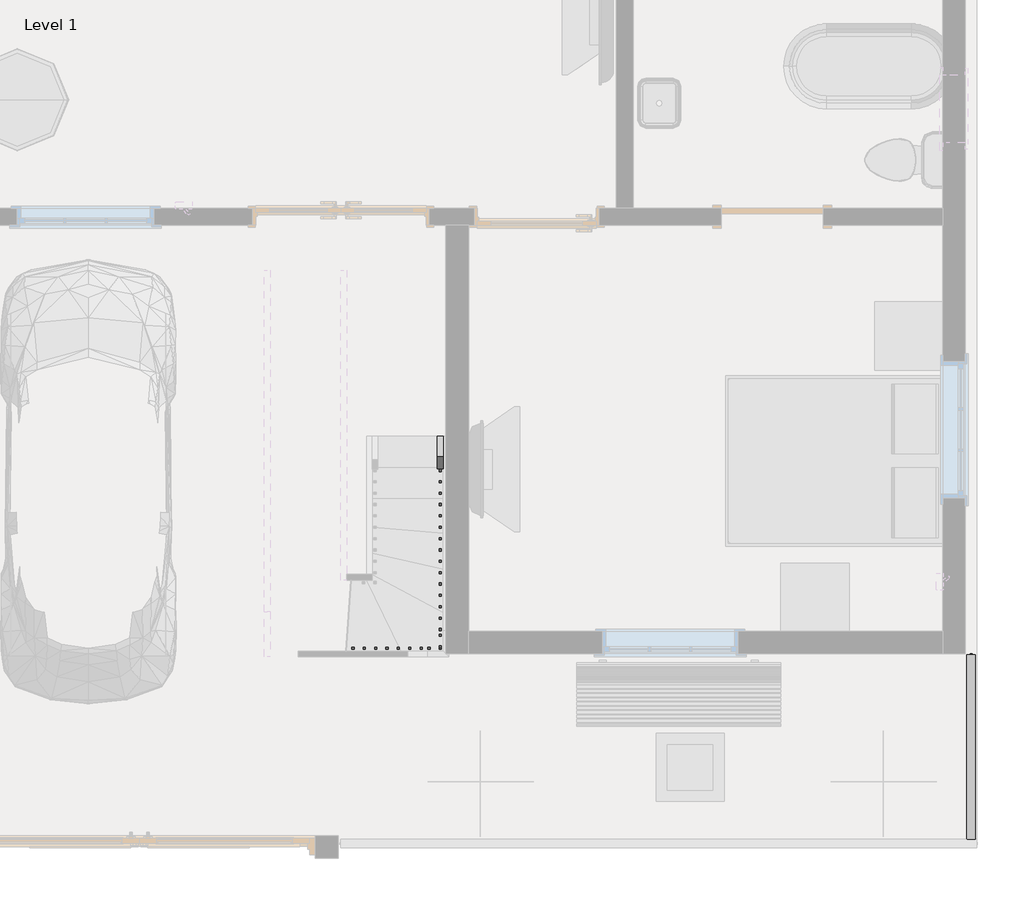
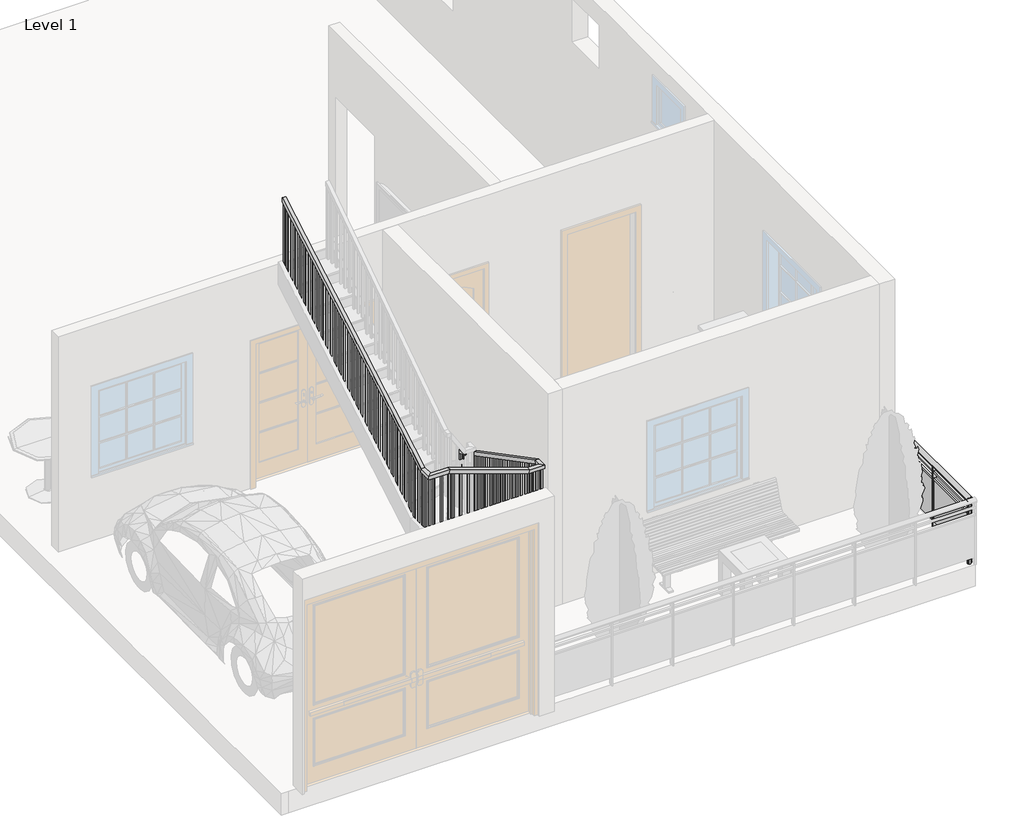
# One storey, part 2 of 3: 2 railings.
"""IFC4 building model written with IfcOpenShell, lengths in millimetres."""

from ifc_helpers import new_model, si_unit, point, frame, origin, origin_with_axes, place, context, project, spatial, polyline, ellipse_curve, trimmed, outline, extrude, faceted_brep, element, save
from ifc_brep_helpers import plane_surface, extruded_surface, advanced_brep

model = new_model("IFC4")

# Units and contexts
model_context = context("Model", 3, world=origin())
ifc_project = project(units=[si_unit("LENGTHUNIT", "METRE", prefix="MILLI")], contexts=[model_context])

# Site, building, storey
site = spatial("IfcSite", under=ifc_project)
building = spatial("IfcBuilding", under=site)
storey = spatial("IfcBuildingStorey", under=building, Name="Level 1", Elevation=0.0)

# Railings
placement = place(None, origin())
element("IfcRailing", 1, ObjectType="Glass Panel - Bottom Fill", at=placement, inside=storey, context=model_context, shape_type="SolidModel", body=[
    advanced_brep(
    [(-6322.409927, -1583.0384156, 914.4), (-6246.209927, -1583.0384156, 914.4), (-6322.409927, 67.9615844, 914.4), (-6246.209927, 67.9615844, 914.4)],
    [
        (0, 1, ellipse_curve(frame((-6284.309927, -1583.0384156, 914.4), z_axis=(0.0, -1.0, 0.0), x_axis=(1.0, 0.0, 0.0)), 38.1, 28.575)),
        (1, 0, ellipse_curve(frame((-6284.309927, -1583.0384156, 914.4), z_axis=(0.0, -1.0, 0.0), x_axis=(1.0, 0.0, 0.0)), 38.1, 28.575)),
        (2, 3, ellipse_curve(frame((-6284.309927, 67.9615844, 914.4), z_axis=(0.0, 1.0, 0.0), x_axis=(1.0, 0.0, 0.0)), 38.1, 28.575)),
        (3, 2, ellipse_curve(frame((-6284.309927, 67.9615844, 914.4), z_axis=(0.0, 1.0, 0.0), x_axis=(1.0, 0.0, 0.0)), 38.1, 28.575)),
        (0, 2),
        (3, 1),
    ],
    [
        plane_surface(frame((-6284.309927, -1583.0384156, 914.4), z_axis=(0.0, -1.0, 0.0), x_axis=(0.0, 0.0, 1.0))),
        plane_surface(frame((-6284.309927, 67.9615844, 914.4), z_axis=(0.0, 1.0, 0.0), x_axis=(0.0, 0.0, 1.0))),
        extruded_surface(trimmed(ellipse_curve(frame((-6284.309927, 67.9615844, 914.4), z_axis=(0.0, -1.0, 0.0), x_axis=(1.0, 0.0, 0.0)), 38.1, 28.575), [point((-6322.409927, 67.9615844, 914.4))], [point((-6246.209927, 67.9615844, 914.4))], True, "CARTESIAN"), (0.0, -1651.0, 0.0), 1651.0),
        extruded_surface(trimmed(ellipse_curve(frame((-6284.309927, 67.9615844, 914.4), z_axis=(0.0, -1.0, 0.0), x_axis=(1.0, 0.0, 0.0)), 38.1, 28.575), [point((-6246.209927, 67.9615844, 914.4))], [point((-6322.409927, 67.9615844, 914.4))], True, "CARTESIAN"), (0.0, -1651.0, 0.0), 1651.0),
    ],
    [
        (0, [[1, 2]]),
        (1, [[3, 4]]),
        (2, [[-1, 5, -4, 6]]),
        (3, [[-2, -6, -3, -5]]),
    ],
),
    extrude(outline(polyline([(-6271.609927, -1583.0384156), (-6297.009927, -1583.0384156), (-6297.009927, 67.9615844), (-6271.609927, 67.9615844), (-6271.609927, -1583.0384156)])), frame((0.0, 0.0, 800.1), z_axis=(0.0, 0.0, 1.0), x_axis=(1.0, 0.0, 0.0)), (0.0, 0.0, 1.0), 25.4),
    extrude(outline(polyline([(-6271.609927, -1583.0384156), (-6297.009927, -1583.0384156), (-6297.009927, 67.9615844), (-6271.609927, 67.9615844), (-6271.609927, -1583.0384156)])), frame((0.0, 0.0, 698.5), z_axis=(0.0, 0.0, 1.0), x_axis=(1.0, 0.0, 0.0)), (0.0, 0.0, 1.0), 25.4),
    extrude(outline(polyline([(-6258.909927, 48.9115844), (-6309.709927, 48.9115844), (-6309.709927, 61.6115844), (-6258.909927, 61.6115844), (-6258.909927, 48.9115844)])), origin_with_axes(), (0.0, 0.0, 1.0), 885.6788223),
    extrude(outline(polyline([(-6290.845084, -757.5384156), (-6290.845084, 55.2615844), (-6284.495084, 55.2615844), (-6284.495084, -757.5384156), (-6290.845084, -757.5384156)])), frame((0.0, 0.0, 101.6), z_axis=(0.0, 0.0, 1.0), x_axis=(1.0, 0.0, 0.0)), (0.0, 0.0, 1.0), 596.9),
    extrude(outline(polyline([(-6258.909927, -763.8884156), (-6309.709927, -763.8884156), (-6309.709927, -751.1884156), (-6258.909927, -751.1884156), (-6258.909927, -763.8884156)])), origin_with_axes(), (0.0, 0.0, 1.0), 885.6788223),
    extrude(outline(polyline([(-6290.845084, -1570.3384156), (-6290.845084, -757.5384156), (-6284.495084, -757.5384156), (-6284.495084, -1570.3384156), (-6290.845084, -1570.3384156)])), frame((0.0, 0.0, 101.6), z_axis=(0.0, 0.0, 1.0), x_axis=(1.0, 0.0, 0.0)), (0.0, 0.0, 1.0), 596.9),
    extrude(outline(polyline([(-6258.909927, -1576.6884156), (-6309.709927, -1576.6884156), (-6309.709927, -1563.9884156), (-6258.909927, -1563.9884156), (-6258.909927, -1576.6884156)])), origin_with_axes(), (0.0, 0.0, 1.0), 885.6788223),
    extrude(outline(polyline([(-6274.784927, 55.2615844), (-6293.834927, 55.2615844), (-6293.834927, 74.3115844), (-6274.784927, 74.3115844), (-6274.784927, 55.2615844)])), origin_with_axes(), (0.0, 0.0, 1.0), 885.6788223),
    extrude(outline(polyline([(-6274.784927, -1589.3884156), (-6293.834927, -1589.3884156), (-6293.834927, -1570.3384156), (-6274.784927, -1570.3384156), (-6274.784927, -1589.3884156)])), origin_with_axes(), (0.0, 0.0, 1.0), 885.6788223),
])
element("IfcRailing", 2, ObjectType="Handrail - Rectangular", at=placement, inside=storey, context=model_context, shape_type="SolidModel", body=[
    faceted_brep([(-11008.709927, 2021.0747681, 1107.1884661), (-11008.709927, 2021.0747681, 1049.8811723), (-11059.509927, 2021.0747681, 1049.8811723), (-11059.509927, 2021.0747681, 1107.1884661), (-11008.709927, 241.9248873, 2036.1046546), (-11008.709927, 229.4614905, 1985.3046546), (-11059.509927, 229.4614905, 1985.3046546), (-11059.509927, 241.9248873, 2036.1046546), (-11008.709927, 100.7187882, 2036.1046546), (-11008.709927, 100.7187882, 1985.3046546), (-11059.509927, 151.5187882, 1985.3046546), (-11059.509927, 151.5187882, 2036.1046546), (-11205.9185931, 100.7187882, 2036.1046546), (-11214.5966373, 100.7187882, 1985.3046546), (-11214.5966373, 151.5187882, 1985.3046546), (-11205.9185931, 151.5187882, 2036.1046546), (-12274.7947104, 100.7187882, 2412.269093), (-12283.4727547, 100.7187882, 2361.469093), (-12283.4727547, 151.5187882, 2361.469093), (-12274.7947104, 151.5187882, 2412.269093), (-12558.109927, 100.7187882, 2412.269093), (-12558.109927, 100.7187882, 2361.469093), (-12507.309927, 151.5187882, 2361.469093), (-12507.309927, 151.5187882, 2412.269093), (-12558.109927, 281.7971454, 2412.269093), (-12558.109927, 295.524936, 2361.469093), (-12507.309927, 295.524936, 2361.469093), (-12507.309927, 281.7971454, 2412.269093), (-12558.109927, 3510.3281176, 4294.6349858), (-12507.309927, 3510.3281176, 4294.6349858), (-12507.309927, 3510.3281176, 4235.8311212), (-12558.109927, 3510.3281176, 4235.8311212)], [[[0, 1, 2, 3]], [[1, 0, 4, 5]], [[2, 1, 5, 6]], [[3, 2, 6, 7]], [[0, 3, 7, 4]], [[5, 4, 8, 9]], [[6, 5, 9, 10]], [[7, 6, 10, 11]], [[4, 7, 11, 8]], [[9, 8, 12, 13]], [[10, 9, 13, 14]], [[11, 10, 14, 15]], [[8, 11, 15, 12]], [[13, 12, 16, 17]], [[14, 13, 17, 18]], [[15, 14, 18, 19]], [[12, 15, 19, 16]], [[17, 16, 20, 21]], [[18, 17, 21, 22]], [[19, 18, 22, 23]], [[16, 19, 23, 20]], [[21, 20, 24, 25]], [[22, 21, 25, 26]], [[23, 22, 26, 27]], [[20, 23, 27, 24]], [[28, 29, 30, 31]], [[25, 24, 28, 31]], [[26, 25, 31, 30]], [[27, 26, 30, 29]], [[24, 27, 29, 28]]]),
    extrude(outline(polyline([(3440.9221454, 4195.3645945), (3440.9221454, 3217.3333333), (3421.8721454, 3217.3333333), (3421.8721454, 4184.2576637), (3440.9221454, 4195.3645945)])), frame((-12542.234927, 0.0, 0.0), z_axis=(1.0, 0.0, 0.0), x_axis=(0.0, 1.0, 0.0)), (0.0, 0.0, 1.0), 19.05),
    extrude(outline(polyline([(3339.3221454, 4136.12763), (3339.3221454, 3217.3333333), (3320.2721454, 3217.3333333), (3320.2721454, 4125.0206991), (3339.3221454, 4136.12763)])), frame((-12542.234927, 0.0, 0.0), z_axis=(1.0, 0.0, 0.0), x_axis=(0.0, 1.0, 0.0)), (0.0, 0.0, 1.0), 19.05),
    extrude(outline(polyline([(3237.7221454, 4076.8906654), (3237.7221454, 3048.0), (3218.6721454, 3048.0), (3218.6721454, 4065.7837346), (3237.7221454, 4076.8906654)])), frame((-12542.234927, 0.0, 0.0), z_axis=(1.0, 0.0, 0.0), x_axis=(0.0, 1.0, 0.0)), (0.0, 0.0, 1.0), 19.05),
    extrude(outline(polyline([(3136.1221454, 4017.6537009), (3136.1221454, 3048.0), (3117.0721454, 3048.0), (3117.0721454, 4006.5467701), (3136.1221454, 4017.6537009)])), frame((-12542.234927, 0.0, 0.0), z_axis=(1.0, 0.0, 0.0), x_axis=(0.0, 1.0, 0.0)), (0.0, 0.0, 1.0), 19.05),
    extrude(outline(polyline([(3034.5221454, 3958.4167364), (3034.5221454, 3048.0), (3015.4721454, 3048.0), (3015.4721454, 3947.3098055), (3034.5221454, 3958.4167364)])), frame((-12542.234927, 0.0, 0.0), z_axis=(1.0, 0.0, 0.0), x_axis=(0.0, 1.0, 0.0)), (0.0, 0.0, 1.0), 19.05),
    extrude(outline(polyline([(2932.9221454, 3899.1797718), (2932.9221454, 2878.6666667), (2913.8721454, 2878.6666667), (2913.8721454, 3888.072841), (2932.9221454, 3899.1797718)])), frame((-12542.234927, 0.0, 0.0), z_axis=(1.0, 0.0, 0.0), x_axis=(0.0, 1.0, 0.0)), (0.0, 0.0, 1.0), 19.05),
    extrude(outline(polyline([(2831.3221454, 3839.9428073), (2831.3221454, 2878.6666667), (2812.2721454, 2878.6666667), (2812.2721454, 3828.8358764), (2831.3221454, 3839.9428073)])), frame((-12542.234927, 0.0, 0.0), z_axis=(1.0, 0.0, 0.0), x_axis=(0.0, 1.0, 0.0)), (0.0, 0.0, 1.0), 19.05),
    extrude(outline(polyline([(2729.7221454, 3780.7058428), (2729.7221454, 2878.6666667), (2710.6721454, 2878.6666667), (2710.6721454, 3769.5989119), (2729.7221454, 3780.7058428)])), frame((-12542.234927, 0.0, 0.0), z_axis=(1.0, 0.0, 0.0), x_axis=(0.0, 1.0, 0.0)), (0.0, 0.0, 1.0), 19.05),
    extrude(outline(polyline([(2628.1221454, 3721.4688782), (2628.1221454, 2709.3333333), (2609.0721454, 2709.3333333), (2609.0721454, 3710.3619474), (2628.1221454, 3721.4688782)])), frame((-12542.234927, 0.0, 0.0), z_axis=(1.0, 0.0, 0.0), x_axis=(0.0, 1.0, 0.0)), (0.0, 0.0, 1.0), 19.05),
    extrude(outline(polyline([(2526.5221454, 3662.2319137), (2526.5221454, 2709.3333333), (2507.4721454, 2709.3333333), (2507.4721454, 3651.1249828), (2526.5221454, 3662.2319137)])), frame((-12542.234927, 0.0, 0.0), z_axis=(1.0, 0.0, 0.0), x_axis=(0.0, 1.0, 0.0)), (0.0, 0.0, 1.0), 19.05),
    extrude(outline(polyline([(2424.9221454, 3602.9949491), (2424.9221454, 2709.3333333), (2405.8721454, 2709.3333333), (2405.8721454, 3591.8880183), (2424.9221454, 3602.9949491)])), frame((-12542.234927, 0.0, 0.0), z_axis=(1.0, 0.0, 0.0), x_axis=(0.0, 1.0, 0.0)), (0.0, 0.0, 1.0), 19.05),
    extrude(outline(polyline([(2323.3221454, 3543.7579846), (2323.3221454, 2540.0), (2304.2721454, 2540.0), (2304.2721454, 3532.6510537), (2323.3221454, 3543.7579846)])), frame((-12542.234927, 0.0, 0.0), z_axis=(1.0, 0.0, 0.0), x_axis=(0.0, 1.0, 0.0)), (0.0, 0.0, 1.0), 19.05),
    extrude(outline(polyline([(2221.7221454, 3484.5210201), (2221.7221454, 2540.0), (2202.6721454, 2540.0), (2202.6721454, 3473.4140892), (2221.7221454, 3484.5210201)])), frame((-12542.234927, 0.0, 0.0), z_axis=(1.0, 0.0, 0.0), x_axis=(0.0, 1.0, 0.0)), (0.0, 0.0, 1.0), 19.05),
    extrude(outline(polyline([(2120.1221454, 3425.2840555), (2120.1221454, 2540.0), (2101.0721454, 2540.0), (2101.0721454, 3414.1771247), (2120.1221454, 3425.2840555)])), frame((-12542.234927, 0.0, 0.0), z_axis=(1.0, 0.0, 0.0), x_axis=(0.0, 1.0, 0.0)), (0.0, 0.0, 1.0), 19.05),
    extrude(outline(polyline([(2018.5221454, 3366.047091), (2018.5221454, 2370.6666667), (1999.4721454, 2370.6666667), (1999.4721454, 3354.9401601), (2018.5221454, 3366.047091)])), frame((-12542.234927, 0.0, 0.0), z_axis=(1.0, 0.0, 0.0), x_axis=(0.0, 1.0, 0.0)), (0.0, 0.0, 1.0), 19.05),
    extrude(outline(polyline([(1916.9221454, 3306.8101264), (1916.9221454, 2370.6666667), (1897.8721454, 2370.6666667), (1897.8721454, 3295.7031956), (1916.9221454, 3306.8101264)])), frame((-12542.234927, 0.0, 0.0), z_axis=(1.0, 0.0, 0.0), x_axis=(0.0, 1.0, 0.0)), (0.0, 0.0, 1.0), 19.05),
    extrude(outline(polyline([(1815.3221454, 3247.5731619), (1815.3221454, 2201.3333333), (1796.2721454, 2201.3333333), (1796.2721454, 3236.466231), (1815.3221454, 3247.5731619)])), frame((-12542.234927, 0.0, 0.0), z_axis=(1.0, 0.0, 0.0), x_axis=(0.0, 1.0, 0.0)), (0.0, 0.0, 1.0), 19.05),
    extrude(outline(polyline([(1713.7221454, 3188.3361974), (1713.7221454, 2201.3333333), (1694.6721454, 2201.3333333), (1694.6721454, 3177.2292665), (1713.7221454, 3188.3361974)])), frame((-12542.234927, 0.0, 0.0), z_axis=(1.0, 0.0, 0.0), x_axis=(0.0, 1.0, 0.0)), (0.0, 0.0, 1.0), 19.05),
    extrude(outline(polyline([(1612.1221454, 3129.0992328), (1612.1221454, 2201.3333333), (1593.0721454, 2201.3333333), (1593.0721454, 3117.992302), (1612.1221454, 3129.0992328)])), frame((-12542.234927, 0.0, 0.0), z_axis=(1.0, 0.0, 0.0), x_axis=(0.0, 1.0, 0.0)), (0.0, 0.0, 1.0), 19.05),
    extrude(outline(polyline([(1510.5221454, 3069.8622683), (1510.5221454, 2032.0), (1491.4721454, 2032.0), (1491.4721454, 3058.7553374), (1510.5221454, 3069.8622683)])), frame((-12542.234927, 0.0, 0.0), z_axis=(1.0, 0.0, 0.0), x_axis=(0.0, 1.0, 0.0)), (0.0, 0.0, 1.0), 19.05),
    extrude(outline(polyline([(1408.9221454, 3010.6253037), (1408.9221454, 2032.0), (1389.8721454, 2032.0), (1389.8721454, 2999.5183729), (1408.9221454, 3010.6253037)])), frame((-12542.234927, 0.0, 0.0), z_axis=(1.0, 0.0, 0.0), x_axis=(0.0, 1.0, 0.0)), (0.0, 0.0, 1.0), 19.05),
    extrude(outline(polyline([(1307.3221454, 2951.3883392), (1307.3221454, 2032.0), (1288.2721454, 2032.0), (1288.2721454, 2940.2814083), (1307.3221454, 2951.3883392)])), frame((-12542.234927, 0.0, 0.0), z_axis=(1.0, 0.0, 0.0), x_axis=(0.0, 1.0, 0.0)), (0.0, 0.0, 1.0), 19.05),
    extrude(outline(polyline([(1205.7221454, 2892.1513747), (1205.7221454, 1862.6666667), (1186.6721454, 1862.6666667), (1186.6721454, 2881.0444438), (1205.7221454, 2892.1513747)])), frame((-12542.234927, 0.0, 0.0), z_axis=(1.0, 0.0, 0.0), x_axis=(0.0, 1.0, 0.0)), (0.0, 0.0, 1.0), 19.05),
    extrude(outline(polyline([(1104.1221454, 2832.9144101), (1104.1221454, 1862.6666667), (1085.0721454, 1862.6666667), (1085.0721454, 2821.8074793), (1104.1221454, 2832.9144101)])), frame((-12542.234927, 0.0, 0.0), z_axis=(1.0, 0.0, 0.0), x_axis=(0.0, 1.0, 0.0)), (0.0, 0.0, 1.0), 19.05),
    extrude(outline(polyline([(1002.5221454, 2773.6774456), (1002.5221454, 1862.6666667), (983.4721454, 1862.6666667), (983.4721454, 2762.5705147), (1002.5221454, 2773.6774456)])), frame((-12542.234927, 0.0, 0.0), z_axis=(1.0, 0.0, 0.0), x_axis=(0.0, 1.0, 0.0)), (0.0, 0.0, 1.0), 19.05),
    extrude(outline(polyline([(900.9221454, 2714.440481), (900.9221454, 1693.3333333), (881.8721454, 1693.3333333), (881.8721454, 2703.3335502), (900.9221454, 2714.440481)])), frame((-12542.234927, 0.0, 0.0), z_axis=(1.0, 0.0, 0.0), x_axis=(0.0, 1.0, 0.0)), (0.0, 0.0, 1.0), 19.05),
    extrude(outline(polyline([(799.3221454, 2655.2035165), (799.3221454, 1693.3333333), (780.2721454, 1693.3333333), (780.2721454, 2644.0965856), (799.3221454, 2655.2035165)])), frame((-12542.234927, 0.0, 0.0), z_axis=(1.0, 0.0, 0.0), x_axis=(0.0, 1.0, 0.0)), (0.0, 0.0, 1.0), 19.05),
    extrude(outline(polyline([(697.7221454, 2595.966552), (697.7221454, 1693.3333333), (678.6721454, 1693.3333333), (678.6721454, 2584.8596211), (697.7221454, 2595.966552)])), frame((-12542.234927, 0.0, 0.0), z_axis=(1.0, 0.0, 0.0), x_axis=(0.0, 1.0, 0.0)), (0.0, 0.0, 1.0), 19.05),
    extrude(outline(polyline([(596.1221454, 2536.7295874), (596.1221454, 1524.0), (577.0721454, 1524.0), (577.0721454, 2525.6226566), (596.1221454, 2536.7295874)])), frame((-12542.234927, 0.0, 0.0), z_axis=(1.0, 0.0, 0.0), x_axis=(0.0, 1.0, 0.0)), (0.0, 0.0, 1.0), 19.05),
    extrude(outline(polyline([(494.5221454, 2477.4926229), (494.5221454, 1524.0), (475.4721454, 1524.0), (475.4721454, 2466.385692), (494.5221454, 2477.4926229)])), frame((-12542.234927, 0.0, 0.0), z_axis=(1.0, 0.0, 0.0), x_axis=(0.0, 1.0, 0.0)), (0.0, 0.0, 1.0), 19.05),
    extrude(outline(polyline([(392.9221454, 2418.2556583), (392.9221454, 1524.0), (373.8721454, 1524.0), (373.8721454, 2407.1487275), (392.9221454, 2418.2556583)])), frame((-12542.234927, 0.0, 0.0), z_axis=(1.0, 0.0, 0.0), x_axis=(0.0, 1.0, 0.0)), (0.0, 0.0, 1.0), 19.05),
    extrude(outline(polyline([(-12542.234927, 218.1937882), (-12542.234927, 237.2437882), (-12523.184927, 237.2437882), (-12523.184927, 218.1937882), (-12542.234927, 218.1937882)])), frame((0.0, 0.0, 1524.0), z_axis=(0.0, 0.0, 1.0), x_axis=(1.0, 0.0, 0.0)), (0.0, 0.0, 1.0), 837.469093),
    extrude(outline(polyline([(-12468.4697104, 116.5937882), (-12487.5197104, 116.5937882), (-12487.5197104, 135.6437882), (-12468.4697104, 135.6437882), (-12468.4697104, 116.5937882)])), frame((0.0, 0.0, 1524.0), z_axis=(0.0, 0.0, 1.0), x_axis=(1.0, 0.0, 0.0)), (0.0, 0.0, 1.0), 837.469093),
    extrude(outline(polyline([(-12366.8697104, 116.5937882), (-12385.9197104, 116.5937882), (-12385.9197104, 135.6437882), (-12366.8697104, 135.6437882), (-12366.8697104, 116.5937882)])), frame((0.0, 0.0, 1524.0), z_axis=(0.0, 0.0, 1.0), x_axis=(1.0, 0.0, 0.0)), (0.0, 0.0, 1.0), 837.469093),
    extrude(outline(polyline([(2343.15872, -12231.4435931), (1354.6666667, -12231.4435931), (1354.6666667, -12212.3935931), (2336.454545, -12212.3935931), (2343.15872, -12231.4435931)])), frame((0.0, 116.5937882, 0.0), z_axis=(0.0, 1.0, 0.0), x_axis=(0.0, 0.0, 1.0)), (0.0, 0.0, 1.0), 19.05),
    extrude(outline(polyline([(2307.40312, -12129.8435931), (1354.6666667, -12129.8435931), (1354.6666667, -12110.7935931), (2300.698945, -12110.7935931), (2307.40312, -12129.8435931)])), frame((0.0, 116.5937882, 0.0), z_axis=(0.0, 1.0, 0.0), x_axis=(0.0, 0.0, 1.0)), (0.0, 0.0, 1.0), 19.05),
    extrude(outline(polyline([(2271.6475199, -12028.2435931), (1354.6666667, -12028.2435931), (1354.6666667, -12009.1935931), (2264.9433449, -12009.1935931), (2271.6475199, -12028.2435931)])), frame((0.0, 116.5937882, 0.0), z_axis=(0.0, 1.0, 0.0), x_axis=(0.0, 0.0, 1.0)), (0.0, 0.0, 1.0), 19.05),
    extrude(outline(polyline([(2235.8919199, -11926.6435931), (1354.6666667, -11926.6435931), (1354.6666667, -11907.5935931), (2229.1877449, -11907.5935931), (2235.8919199, -11926.6435931)])), frame((0.0, 116.5937882, 0.0), z_axis=(0.0, 1.0, 0.0), x_axis=(0.0, 0.0, 1.0)), (0.0, 0.0, 1.0), 19.05),
    extrude(outline(polyline([(2200.1363199, -11825.0435931), (1185.3333333, -11825.0435931), (1185.3333333, -11805.9935931), (2193.4321449, -11805.9935931), (2200.1363199, -11825.0435931)])), frame((0.0, 116.5937882, 0.0), z_axis=(0.0, 1.0, 0.0), x_axis=(0.0, 0.0, 1.0)), (0.0, 0.0, 1.0), 19.05),
    extrude(outline(polyline([(2164.3807198, -11723.4435931), (1185.3333333, -11723.4435931), (1185.3333333, -11704.3935931), (2157.6765448, -11704.3935931), (2164.3807198, -11723.4435931)])), frame((0.0, 116.5937882, 0.0), z_axis=(0.0, 1.0, 0.0), x_axis=(0.0, 0.0, 1.0)), (0.0, 0.0, 1.0), 19.05),
    extrude(outline(polyline([(2128.6251198, -11621.8435931), (1185.3333333, -11621.8435931), (1185.3333333, -11602.7935931), (2121.9209448, -11602.7935931), (2128.6251198, -11621.8435931)])), frame((0.0, 116.5937882, 0.0), z_axis=(0.0, 1.0, 0.0), x_axis=(0.0, 0.0, 1.0)), (0.0, 0.0, 1.0), 19.05),
    extrude(outline(polyline([(2092.8695198, -11520.2435931), (1185.3333333, -11520.2435931), (1185.3333333, -11501.1935931), (2086.1653448, -11501.1935931), (2092.8695198, -11520.2435931)])), frame((0.0, 116.5937882, 0.0), z_axis=(0.0, 1.0, 0.0), x_axis=(0.0, 0.0, 1.0)), (0.0, 0.0, 1.0), 19.05),
    extrude(outline(polyline([(2057.1139197, -11418.6435931), (1185.3333333, -11418.6435931), (1185.3333333, -11399.5935931), (2050.4097447, -11399.5935931), (2057.1139197, -11418.6435931)])), frame((0.0, 116.5937882, 0.0), z_axis=(0.0, 1.0, 0.0), x_axis=(0.0, 0.0, 1.0)), (0.0, 0.0, 1.0), 19.05),
    extrude(outline(polyline([(2021.3583197, -11317.0435931), (1016.0, -11317.0435931), (1016.0, -11297.9935931), (2014.6541447, -11297.9935931), (2021.3583197, -11317.0435931)])), frame((0.0, 116.5937882, 0.0), z_axis=(0.0, 1.0, 0.0), x_axis=(0.0, 0.0, 1.0)), (0.0, 0.0, 1.0), 19.05),
    extrude(outline(polyline([(-11126.184927, 116.5937882), (-11145.234927, 116.5937882), (-11145.234927, 135.6437882), (-11126.184927, 135.6437882), (-11126.184927, 116.5937882)])), frame((0.0, 0.0, 1016.0), z_axis=(0.0, 0.0, 1.0), x_axis=(1.0, 0.0, 0.0)), (0.0, 0.0, 1.0), 969.3046546),
    extrude(outline(polyline([(-11024.584927, 149.8498873), (-11024.584927, 130.7998873), (-11043.634927, 130.7998873), (-11043.634927, 149.8498873), (-11024.584927, 149.8498873)])), frame((0.0, 0.0, 1016.0), z_axis=(0.0, 0.0, 1.0), x_axis=(1.0, 0.0, 0.0)), (0.0, 0.0, 1.0), 969.3046546),
    extrude(outline(polyline([(303.3997681, 1946.7005641), (303.3997681, 1016.0), (284.3497681, 1016.0), (284.3497681, 1956.6468051), (303.3997681, 1946.7005641)])), frame((-11043.634927, 0.0, 0.0), z_axis=(1.0, 0.0, 0.0), x_axis=(0.0, 1.0, 0.0)), (0.0, 0.0, 1.0), 19.05),
    extrude(outline(polyline([(404.9997681, 1893.6539457), (404.9997681, 1016.0), (385.9497681, 1016.0), (385.9497681, 1903.6001867), (404.9997681, 1893.6539457)])), frame((-11043.634927, 0.0, 0.0), z_axis=(1.0, 0.0, 0.0), x_axis=(0.0, 1.0, 0.0)), (0.0, 0.0, 1.0), 19.05),
    extrude(outline(polyline([(506.5997681, 1840.6073274), (506.5997681, 846.6666667), (487.5497681, 846.6666667), (487.5497681, 1850.5535683), (506.5997681, 1840.6073274)])), frame((-11043.634927, 0.0, 0.0), z_axis=(1.0, 0.0, 0.0), x_axis=(0.0, 1.0, 0.0)), (0.0, 0.0, 1.0), 19.05),
    extrude(outline(polyline([(608.1997681, 1787.560709), (608.1997681, 846.6666667), (589.1497681, 846.6666667), (589.1497681, 1797.5069499), (608.1997681, 1787.560709)])), frame((-11043.634927, 0.0, 0.0), z_axis=(1.0, 0.0, 0.0), x_axis=(0.0, 1.0, 0.0)), (0.0, 0.0, 1.0), 19.05),
    extrude(outline(polyline([(709.7997681, 1734.5140906), (709.7997681, 846.6666667), (690.7497681, 846.6666667), (690.7497681, 1744.4603316), (709.7997681, 1734.5140906)])), frame((-11043.634927, 0.0, 0.0), z_axis=(1.0, 0.0, 0.0), x_axis=(0.0, 1.0, 0.0)), (0.0, 0.0, 1.0), 19.05),
    extrude(outline(polyline([(811.3997681, 1681.4674723), (811.3997681, 846.6666667), (792.3497681, 846.6666667), (792.3497681, 1691.4137132), (811.3997681, 1681.4674723)])), frame((-11043.634927, 0.0, 0.0), z_axis=(1.0, 0.0, 0.0), x_axis=(0.0, 1.0, 0.0)), (0.0, 0.0, 1.0), 19.05),
    extrude(outline(polyline([(912.9997681, 1628.4208539), (912.9997681, 677.3333333), (893.9497681, 677.3333333), (893.9497681, 1638.3670948), (912.9997681, 1628.4208539)])), frame((-11043.634927, 0.0, 0.0), z_axis=(1.0, 0.0, 0.0), x_axis=(0.0, 1.0, 0.0)), (0.0, 0.0, 1.0), 19.05),
    extrude(outline(polyline([(1014.5997681, 1575.3742355), (1014.5997681, 677.3333333), (995.5497681, 677.3333333), (995.5497681, 1585.3204765), (1014.5997681, 1575.3742355)])), frame((-11043.634927, 0.0, 0.0), z_axis=(1.0, 0.0, 0.0), x_axis=(0.0, 1.0, 0.0)), (0.0, 0.0, 1.0), 19.05),
    extrude(outline(polyline([(1116.1997681, 1522.3276171), (1116.1997681, 677.3333333), (1097.1497681, 677.3333333), (1097.1497681, 1532.2738581), (1116.1997681, 1522.3276171)])), frame((-11043.634927, 0.0, 0.0), z_axis=(1.0, 0.0, 0.0), x_axis=(0.0, 1.0, 0.0)), (0.0, 0.0, 1.0), 19.05),
    extrude(outline(polyline([(1217.7997681, 1469.146339), (1217.7997681, 508.0), (1198.7497681, 508.0), (1198.7497681, 1479.0874531), (1217.7997681, 1469.146339)])), frame((-11043.634927, 0.0, 0.0), z_axis=(1.0, 0.0, 0.0), x_axis=(0.0, 1.0, 0.0)), (0.0, 0.0, 1.0), 19.05),
    extrude(outline(polyline([(1319.3997681, 1416.2343804), (1319.3997681, 508.0), (1300.3497681, 508.0), (1300.3497681, 1426.1806213), (1319.3997681, 1416.2343804)])), frame((-11043.634927, 0.0, 0.0), z_axis=(1.0, 0.0, 0.0), x_axis=(0.0, 1.0, 0.0)), (0.0, 0.0, 1.0), 19.05),
    extrude(outline(polyline([(1420.9997681, 1363.187762), (1420.9997681, 508.0), (1401.9497681, 508.0), (1401.9497681, 1373.134003), (1420.9997681, 1363.187762)])), frame((-11043.634927, 0.0, 0.0), z_axis=(1.0, 0.0, 0.0), x_axis=(0.0, 1.0, 0.0)), (0.0, 0.0, 1.0), 19.05),
    extrude(outline(polyline([(1522.5997681, 1310.0885121), (1522.5997681, 338.6666667), (1503.5497681, 338.6666667), (1503.5497681, 1320.0296262), (1522.5997681, 1310.0885121)])), frame((-11043.634927, 0.0, 0.0), z_axis=(1.0, 0.0, 0.0), x_axis=(0.0, 1.0, 0.0)), (0.0, 0.0, 1.0), 19.05),
    extrude(outline(polyline([(1624.1997681, 1257.0945253), (1624.1997681, 338.6666667), (1605.1497681, 338.6666667), (1605.1497681, 1267.0407662), (1624.1997681, 1257.0945253)])), frame((-11043.634927, 0.0, 0.0), z_axis=(1.0, 0.0, 0.0), x_axis=(0.0, 1.0, 0.0)), (0.0, 0.0, 1.0), 19.05),
    extrude(outline(polyline([(1725.7997681, 1204.0479069), (1725.7997681, 338.6666667), (1706.7497681, 338.6666667), (1706.7497681, 1213.9941479), (1725.7997681, 1204.0479069)])), frame((-11043.634927, 0.0, 0.0), z_axis=(1.0, 0.0, 0.0), x_axis=(0.0, 1.0, 0.0)), (0.0, 0.0, 1.0), 19.05),
    extrude(outline(polyline([(1827.3997681, 1151.0306852), (1827.3997681, 169.3333333), (1808.3497681, 169.3333333), (1808.3497681, 1160.9717994), (1827.3997681, 1151.0306852)])), frame((-11043.634927, 0.0, 0.0), z_axis=(1.0, 0.0, 0.0), x_axis=(0.0, 1.0, 0.0)), (0.0, 0.0, 1.0), 19.05),
    extrude(outline(polyline([(1928.9997681, 1097.9546702), (1928.9997681, 169.3333333), (1909.9497681, 169.3333333), (1909.9497681, 1107.9009111), (1928.9997681, 1097.9546702)])), frame((-11043.634927, 0.0, 0.0), z_axis=(1.0, 0.0, 0.0), x_axis=(0.0, 1.0, 0.0)), (0.0, 0.0, 1.0), 19.05),
    extrude(outline(polyline([(-12542.234927, 272.2721454), (-12542.234927, 291.3221454), (-12523.184927, 291.3221454), (-12523.184927, 272.2721454), (-12542.234927, 272.2721454)])), frame((0.0, 0.0, 1524.0), z_axis=(0.0, 0.0, 1.0), x_axis=(1.0, 0.0, 0.0)), (0.0, 0.0, 1.0), 837.469093),
    extrude(outline(polyline([(-12523.184927, 116.5937882), (-12542.234927, 116.5937882), (-12542.234927, 135.6437882), (-12523.184927, 135.6437882), (-12523.184927, 116.5937882)])), frame((0.0, 0.0, 1524.0), z_axis=(0.0, 0.0, 1.0), x_axis=(1.0, 0.0, 0.0)), (0.0, 0.0, 1.0), 837.469093),
    extrude(outline(polyline([(2361.767158, -12284.3197104), (1354.6666667, -12284.3197104), (1354.6666667, -12265.2697104), (2355.062983, -12265.2697104), (2361.767158, -12284.3197104)])), frame((0.0, 116.5937882, 0.0), z_axis=(0.0, 1.0, 0.0), x_axis=(0.0, 0.0, 1.0)), (0.0, 0.0, 1.0), 19.05),
    extrude(outline(polyline([(-11196.3935931, 116.5937882), (-11215.4435931, 116.5937882), (-11215.4435931, 135.6437882), (-11196.3935931, 135.6437882), (-11196.3935931, 116.5937882)])), frame((0.0, 0.0, 1016.0), z_axis=(0.0, 0.0, 1.0), x_axis=(1.0, 0.0, 0.0)), (0.0, 0.0, 1.0), 969.3046546),
    extrude(outline(polyline([(-11024.584927, 135.6437882), (-11024.584927, 116.5937882), (-11043.634927, 116.5937882), (-11043.634927, 135.6437882), (-11024.584927, 135.6437882)])), frame((0.0, 0.0, 1016.0), z_axis=(0.0, 0.0, 1.0), x_axis=(1.0, 0.0, 0.0)), (0.0, 0.0, 1.0), 969.3046546),
    extrude(outline(polyline([(251.4498873, 1973.8242403), (251.4498873, 1016.0), (232.3998873, 1016.0), (232.3998873, 1983.7704812), (251.4498873, 1973.8242403)])), frame((-11043.634927, 0.0, 0.0), z_axis=(1.0, 0.0, 0.0), x_axis=(0.0, 1.0, 0.0)), (0.0, 0.0, 1.0), 19.05),
    extrude(outline(polyline([(3510.3281176, 4235.8311212), (3510.3281176, 3217.3333333), (3491.2781176, 3217.3333333), (3491.2781176, 4224.7241904), (3510.3281176, 4235.8311212)])), frame((-12542.234927, 0.0, 0.0), z_axis=(1.0, 0.0, 0.0), x_axis=(0.0, 1.0, 0.0)), (0.0, 0.0, 1.0), 19.05),
    extrude(outline(polyline([(2021.0747681, 1049.8811723), (2021.0747681, 169.3333333), (2002.0247681, 169.3333333), (2002.0247681, 1059.8274132), (2021.0747681, 1049.8811723)])), frame((-11043.634927, 0.0, 0.0), z_axis=(1.0, 0.0, 0.0), x_axis=(0.0, 1.0, 0.0)), (0.0, 0.0, 1.0), 19.05),
])

save(model, "model.ifc")

# Revit data of these elements
# Type "Glass Panel - Bottom Fill"
#   Assembly Code = "C2010400"
#   built-in parameter 1008612 = 0.0416667 (stored number, unit not read)
#   built-in parameter 1008611 = 0.0416667 (stored number, unit not read)
#   built-in parameter 1008609 = 0.333333 (stored number, unit not read)
#   built-in parameter 1008604 = 0.166667 (stored number, unit not read)
#   built-in parameter 1008603 = 0.166667 (stored number, unit not read)
#   Railing Height = 3' - 0"
#   built-in parameter 1008630 = 2
#   built-in parameter 1008610 = 2
#   built-in parameter 1008618 = Baluster - Square : 3/4"
# Type "Handrail - Rectangular"
#   Assembly Code = "C2010400"
#   built-in parameter 1008612 = 0.0416667 (stored number, unit not read)
#   built-in parameter 1008611 = 0.0416667 (stored number, unit not read)
#   built-in parameter 1008609 = 0.333333 (stored number, unit not read)
#   built-in parameter 1008604 = 0.166667 (stored number, unit not read)
#   built-in parameter 1008603 = 0.166667 (stored number, unit not read)
#   Railing Height = 3' - 0"
#   built-in parameter 1008630 = 2
#   built-in parameter 1008610 = 2
#   built-in parameter 1008618 = Baluster - Square : 3/4"
# Element 1 (IfcRailing, "Glass Panel - Bottom Fill")
#   Phase Created = New Construction
#   Materials on its faces: "Glass"
# Element 2 (IfcRailing, "Handrail - Rectangular")
#   Phase Created = New Construction
# Materials
#   "Glass": class "Glass", colour RGB 0 128 192, transparency 0.75, Description = "Soda Lime Glass", Cost = 0
